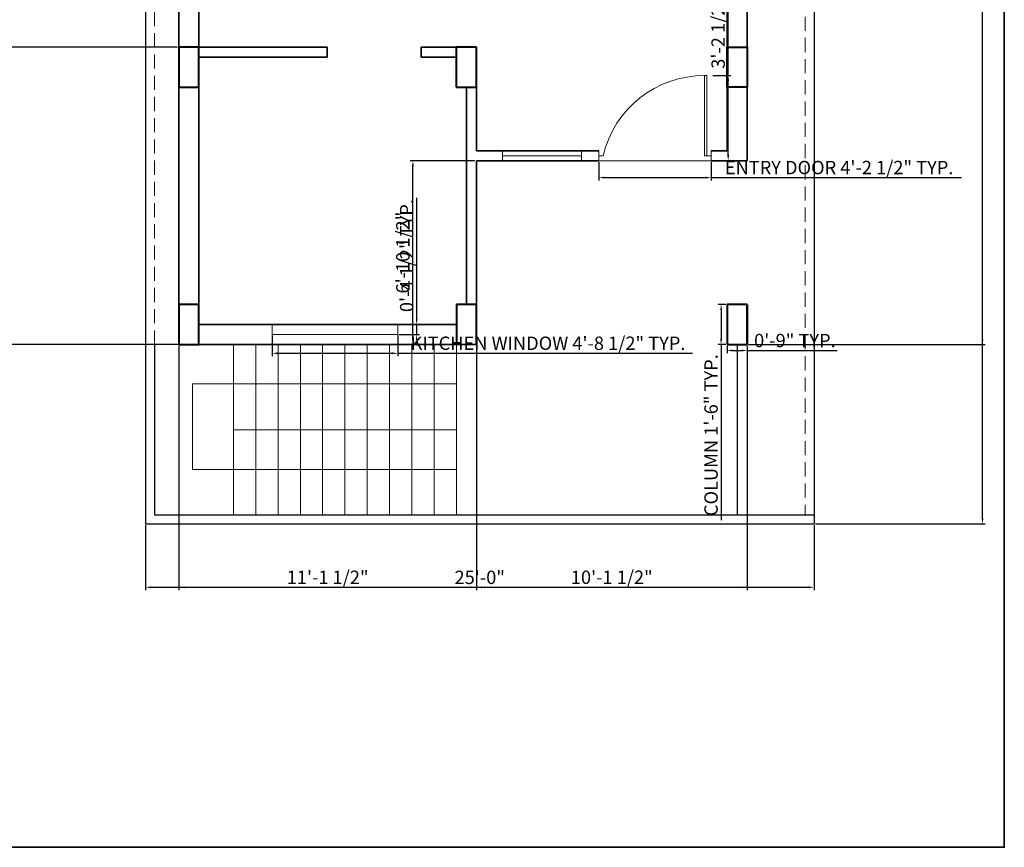
# Model space of a CAD drawing. Units: inches. Extents: x 2656 to 9931, y 1941 to 3068.
# Tile 26 of 46: x 3074 to 3515, y 1941 to 2312. Entities that reach past the tile are written whole.
import ezdxf

# ---------------------------------------------------------------- set-up
doc = ezdxf.new("R2010")
doc.units = ezdxf.units.IN
doc.linetypes.add('DASHED2', pattern=[9.525, 6.35, -3.175])
for name, color, linetype, lineweight in [('A-ANNO-DIMS', 2, 'Continuous', 18), ('A-ANNO-TTLB', 7, 'Continuous', 35), ('A-COLS', 7, 'Continuous', 40), ('A-DOOR', 3, 'Continuous', 18), ('A-FLOR-OVHD', 252, 'DASHED2', 13), ('A-FLOR-STRS', 7, 'Continuous', 18), ('A-GLAZ', 4, 'Continuous', 18), ('A-WALL', 7, 'Continuous', 35), ('C-PROP', 7, 'Continuous', 25)]:
    doc.layers.add(name, color=color, linetype=linetype, lineweight=lineweight)
doc.styles.get("Standard").update_dxf_attribs({"font": 'arial.ttf'})
doc.dimstyles.new('ISO-25', dxfattribs={"dimtxt": 6, "dimasz": 2.5, "dimexe": 1.25, "dimexo": 0.625, "dimtad": 1, "dimdec": 0, "dimlunit": 3, "dimtxsty": 'Standard', "dimcen": 2.5, "dimadec": 0, "dimazin": 0, "dimtfac": 1, "dimtdec": 0, "dimtmove": 0, "dimatfit": 3, "dimfxl": 1, "dimarcsym": 0})

# ---------------------------------------------------------------- blocks, each defined once
blk = doc.blocks.new('DOOR-ENTRY')
for p, q in [((48.56, 38.25), (47.56, 38.25)), ((47.56, 38.25), (47.56, 2.25)), ((48.56, 2.25), (48.56, 38.25)), ((0.04, 2.25), (2.04, 2.25)), ((0.04, 0), (50.56, 0)), ((47.56, 2.25), (48.56, 2.25)), ((50.56, 2.25), (48.56, 2.25))]:
    blk.add_line(p, q)
blk.add_arc((47.56, -8.52), 46.77, 90, 166.6828)
blk = doc.blocks.new('WIN-ENTRY')
for p, q in [((35.5, -0.05), (35.5, 2.2)), ((0.02, -0.05), (35.5, -0.05))]:
    blk.add_line(p, q)
blk = doc.blocks.new('WIN-KITCHEN')
for p, q in [((56.32, 0), (56.32, 4.5)), ((-0.04, 0), (56.32, 0))]:
    blk.add_line(p, q)
blk = doc.blocks.new('STAIR-FRONT')
for p, q in [((28.36, 76.5), (18.36, 76.5)), ((18.36, 76.5), (18.36, 0)), ((28.36, 76.5), (28.36, 0)), ((38.36, 76.5), (38.36, 0)), ((48.36, 76.5), (48.36, 0)), ((58.36, 76.5), (58.36, 0)), ((68.36, 76.5), (68.36, 0)), ((78.36, 76.5), (78.36, 0)), ((88.36, 76.5), (88.36, 0)), ((98.36, 76.5), (98.36, 0)), ((108.36, 76.5), (108.36, 0)), ((118.36, 76.5), (118.36, 0)), ((118.36, 58.83), (-0.04, 58.83)), ((-0.04, 58.83), (-0.04, 20.36)), ((18.36, 0), (18.36, 38.25)), ((18.36, 38.25), (28.36, 38.25)), ((118.36, 38.25), (28.36, 38.25)), ((118.36, 0), (118.36, 38.25)), ((-0.04, 20.36), (118.36, 20.36))]:
    blk.add_line(p, q)
blk = doc.blocks.new('COL-9X18')
for p, q in [((18.05, 9), (0.05, 9)), ((0.05, 9), (0.05, 0)), ((18.05, 0), (18.05, 9)), ((0.05, 0), (18.05, 0))]:
    blk.add_line(p, q)
blk = doc.blocks.new('*D25')
at = {"layer": 'A-ANNO-DIMS', "color": 0, "lineweight": -2, "transparency": 16777216}
for p, q in [((3390.42, 2184.6), (3387.1, 2184.6)), ((3388.35, 2182.1), (3388.35, 2169.1)), ((3390.42, 2166.6), (3387.1, 2166.6)), ((3388.35, 2166.6), (3388.35, 2087.69))]:
    blk.add_line(p, q, dxfattribs=at)
at = {"layer": 'A-ANNO-DIMS', "color": 0, "transparency": 16777216}
for points in [[(3387.93, 2182.1), (3388.76, 2182.1), (3388.35, 2184.6)], [(3387.93, 2169.1), (3388.76, 2169.1), (3388.35, 2166.6)]]:
    blk.add_solid(points, dxfattribs=at)
at = {"layer": 'Defpoints', "color": 0, "transparency": 16777216}
for p in [(3391.05, 2184.6), (3388.35, 2166.6), (3391.05, 2166.6)]:
    blk.add_point(p, dxfattribs=at)
at = {"layer": 'A-ANNO-DIMS', "color": 0, "transparency": 16777216, "insert": (3384.62, 2125.9), "char_height": 6, "attachment_point": 5, "rotation": 90}
blk.add_mtext('COLUMN 1\'-6" TYP.', dxfattribs=at)
blk = doc.blocks.new('*D26')
at = {"layer": 'A-ANNO-DIMS', "color": 0, "lineweight": -2, "transparency": 16777216}
for p, q in [((3391.05, 2165.98), (3391.05, 2162.65)), ((3400.05, 2165.98), (3400.05, 2162.65)), ((3393.55, 2163.9), (3397.55, 2163.9)), ((3400.05, 2163.9), (3440.37, 2163.9))]:
    blk.add_line(p, q, dxfattribs=at)
at = {"layer": 'A-ANNO-DIMS', "color": 0, "transparency": 16777216}
for points in [[(3393.55, 2164.32), (3393.55, 2163.48), (3391.05, 2163.9)], [(3397.55, 2164.32), (3397.55, 2163.48), (3400.05, 2163.9)]]:
    blk.add_solid(points, dxfattribs=at)
at = {"layer": 'Defpoints', "color": 0, "transparency": 16777216}
for p in [(3391.05, 2166.6), (3400.05, 2166.6), (3400.05, 2163.9)]:
    blk.add_point(p, dxfattribs=at)
at = {"layer": 'A-ANNO-DIMS', "color": 0, "transparency": 16777216, "insert": (3421.46, 2167.59), "char_height": 6, "attachment_point": 5}
blk.add_mtext('0\'-9" TYP.', dxfattribs=at)
blk = doc.blocks.new('*D41')
at = {"layer": 'A-ANNO-DIMS', "color": 0, "lineweight": -2, "transparency": 16777216}
for p, q in [((3333.43, 2248.48), (3333.43, 2240.27)), ((3383.95, 2248.48), (3383.95, 2240.27)), ((3335.93, 2241.52), (3381.45, 2241.52)), ((3383.95, 2241.52), (3496.15, 2241.52))]:
    blk.add_line(p, q, dxfattribs=at)
at = {"layer": 'A-ANNO-DIMS', "color": 0, "transparency": 16777216}
for points in [[(3335.93, 2241.94), (3335.93, 2241.11), (3333.43, 2241.52)], [(3381.45, 2241.94), (3381.45, 2241.11), (3383.95, 2241.52)]]:
    blk.add_solid(points, dxfattribs=at)
at = {"layer": 'Defpoints', "color": 0, "transparency": 16777216}
for p in [(3333.43, 2249.1), (3383.95, 2249.1), (3383.95, 2241.52)]:
    blk.add_point(p, dxfattribs=at)
at = {"layer": 'A-ANNO-DIMS', "color": 0, "transparency": 16777216, "insert": (3441.3, 2245.25), "char_height": 6, "attachment_point": 5}
blk.add_mtext('ENTRY DOOR 4\'-2 1/2" TYP.', dxfattribs=at)
blk = doc.blocks.new('*D42')
at = {"layer": 'A-ANNO-DIMS', "color": 0, "lineweight": -2, "transparency": 16777216}
for p, q in [((3391.52, 2287.35), (3391.52, 2341.65)), ((3384.57, 2287.35), (3392.77, 2287.35)), ((3391.52, 2251.6), (3391.52, 2284.85)), ((3384.57, 2249.1), (3392.77, 2249.1))]:
    blk.add_line(p, q, dxfattribs=at)
at = {"layer": 'A-ANNO-DIMS', "color": 0, "transparency": 16777216}
for points in [[(3391.11, 2284.85), (3391.94, 2284.85), (3391.52, 2287.35)], [(3391.11, 2251.6), (3391.94, 2251.6), (3391.52, 2249.1)]]:
    blk.add_solid(points, dxfattribs=at)
at = {"layer": 'Defpoints', "color": 0, "transparency": 16777216}
for p in [(3383.95, 2287.35), (3391.52, 2287.35), (3383.95, 2249.1)]:
    blk.add_point(p, dxfattribs=at)
at = {"layer": 'A-ANNO-DIMS', "color": 0, "transparency": 16777216, "insert": (3387.79, 2315.75), "char_height": 6, "attachment_point": 5, "rotation": 90}
blk.add_mtext('3\'-2 1/2" TYP.', dxfattribs=at)
blk = doc.blocks.new('*D51')
at = {"layer": 'A-ANNO-DIMS', "color": 0, "lineweight": -2, "transparency": 16777216}
for p, q in [((3186.95, 2170.48), (3186.95, 2161.4)), ((3243.31, 2170.48), (3243.31, 2161.4)), ((3189.45, 2162.65), (3240.81, 2162.65)), ((3243.31, 2162.65), (3375.57, 2162.65))]:
    blk.add_line(p, q, dxfattribs=at)
at = {"layer": 'A-ANNO-DIMS', "color": 0, "transparency": 16777216}
for points in [[(3189.45, 2163.06), (3189.45, 2162.23), (3186.95, 2162.65)], [(3240.81, 2163.06), (3240.81, 2162.23), (3243.31, 2162.65)]]:
    blk.add_solid(points, dxfattribs=at)
at = {"layer": 'Defpoints', "color": 0, "transparency": 16777216}
for p in [(3186.95, 2171.1), (3243.31, 2171.1), (3243.31, 2162.65)]:
    blk.add_point(p, dxfattribs=at)
at = {"layer": 'A-ANNO-DIMS', "color": 0, "transparency": 16777216, "insert": (3310.69, 2166.38), "char_height": 6, "attachment_point": 5}
blk.add_mtext('KITCHEN WINDOW 4\'-8 1/2" TYP.', dxfattribs=at)
blk = doc.blocks.new('*D52')
at = {"layer": 'A-ANNO-DIMS', "color": 0, "lineweight": -2, "transparency": 16777216}
for p, q in [((3251.76, 2178.1), (3251.76, 2232.4)), ((3243.93, 2175.6), (3253.01, 2175.6)), ((3251.76, 2171.1), (3251.76, 2175.6)), ((3243.93, 2171.1), (3253.01, 2171.1)), ((3251.76, 2168.6), (3251.76, 2166.1))]:
    blk.add_line(p, q, dxfattribs=at)
at = {"layer": 'A-ANNO-DIMS', "color": 0, "transparency": 16777216}
for points in [[(3251.34, 2178.1), (3252.18, 2178.1), (3251.76, 2175.6)], [(3251.34, 2168.6), (3252.18, 2168.6), (3251.76, 2171.1)]]:
    blk.add_solid(points, dxfattribs=at)
at = {"layer": 'Defpoints', "color": 0, "transparency": 16777216}
for p in [(3243.31, 2175.6), (3251.76, 2175.6), (3243.31, 2171.1)]:
    blk.add_point(p, dxfattribs=at)
at = {"layer": 'A-ANNO-DIMS', "color": 0, "transparency": 16777216, "insert": (3248.03, 2206.5), "char_height": 6, "attachment_point": 5, "rotation": 90}
blk.add_mtext('0\'-4 1/2" TYP.', dxfattribs=at)
blk = doc.blocks.new('*D66')
at = {"layer": 'A-ANNO-DIMS', "color": 0, "lineweight": -2, "transparency": 16777216}
for p, q in [((3400.67, 2623.6), (3506.9, 2623.6)), ((3505.65, 2169.1), (3505.65, 2621.1)), ((3400.67, 2166.6), (3506.9, 2166.6))]:
    blk.add_line(p, q, dxfattribs=at)
at = {"layer": 'A-ANNO-DIMS', "color": 0, "transparency": 16777216}
for points in [[(3505.23, 2621.1), (3506.07, 2621.1), (3505.65, 2623.6)], [(3505.23, 2169.1), (3506.07, 2169.1), (3505.65, 2166.6)]]:
    blk.add_solid(points, dxfattribs=at)
at = {"layer": 'Defpoints', "color": 0, "transparency": 16777216}
for p in [(3400.05, 2623.6), (3505.65, 2623.6), (3400.05, 2166.6)]:
    blk.add_point(p, dxfattribs=at)
at = {"layer": 'A-ANNO-DIMS', "color": 0, "transparency": 16777216, "insert": (3501.96, 2395.1), "char_height": 6, "attachment_point": 5, "rotation": 90}
blk.add_mtext('38\'-1"', dxfattribs=at)
blk = doc.blocks.new('*D67')
at = {"layer": 'A-ANNO-DIMS', "color": 0, "lineweight": -2, "transparency": 16777216}
for p, q in [((3145.05, 2165.98), (3145.05, 2056.35)), ((3278.55, 2165.98), (3278.55, 2056.35)), ((3147.55, 2057.6), (3276.05, 2057.6))]:
    blk.add_line(p, q, dxfattribs=at)
at = {"layer": 'A-ANNO-DIMS', "color": 0, "transparency": 16777216}
for points in [[(3147.55, 2058.02), (3147.55, 2057.18), (3145.05, 2057.6)], [(3276.05, 2058.02), (3276.05, 2057.18), (3278.55, 2057.6)]]:
    blk.add_solid(points, dxfattribs=at)
at = {"layer": 'Defpoints', "color": 0, "transparency": 16777216}
for p in [(3145.05, 2166.6), (3278.55, 2166.6), (3278.55, 2057.6)]:
    blk.add_point(p, dxfattribs=at)
at = {"layer": 'A-ANNO-DIMS', "color": 0, "transparency": 16777216, "insert": (3211.8, 2061.33), "char_height": 6, "attachment_point": 5}
blk.add_mtext('11\'-1 1/2"', dxfattribs=at)
blk = doc.blocks.new('*D68')
at = {"layer": 'A-ANNO-DIMS', "color": 0, "lineweight": -2, "transparency": 16777216}
for p, q in [((3278.55, 2165.98), (3278.55, 2056.35)), ((3400.05, 2165.98), (3400.05, 2056.35)), ((3281.05, 2057.6), (3397.55, 2057.6))]:
    blk.add_line(p, q, dxfattribs=at)
at = {"layer": 'A-ANNO-DIMS', "color": 0, "transparency": 16777216}
for points in [[(3281.05, 2058.02), (3281.05, 2057.18), (3278.55, 2057.6)], [(3397.55, 2058.02), (3397.55, 2057.18), (3400.05, 2057.6)]]:
    blk.add_solid(points, dxfattribs=at)
at = {"layer": 'Defpoints', "color": 0, "transparency": 16777216}
for p in [(3278.55, 2166.6), (3400.05, 2166.6), (3400.05, 2057.6)]:
    blk.add_point(p, dxfattribs=at)
at = {"layer": 'A-ANNO-DIMS', "color": 0, "transparency": 16777216, "insert": (3339.3, 2061.33), "char_height": 6, "attachment_point": 5}
blk.add_mtext('10\'-1 1/2"', dxfattribs=at)
blk = doc.blocks.new('*D69')
at = {"layer": 'A-ANNO-DIMS', "color": 0, "lineweight": -2, "transparency": 16777216}
for p, q in [((3144.42, 2300.1), (3052.46, 2300.1)), ((3053.71, 2169.1), (3053.71, 2297.6)), ((3144.42, 2166.6), (3052.46, 2166.6))]:
    blk.add_line(p, q, dxfattribs=at)
at = {"layer": 'A-ANNO-DIMS', "color": 0, "transparency": 16777216}
for points in [[(3053.3, 2297.6), (3054.13, 2297.6), (3053.71, 2300.1)], [(3053.3, 2169.1), (3054.13, 2169.1), (3053.71, 2166.6)]]:
    blk.add_solid(points, dxfattribs=at)
at = {"layer": 'Defpoints', "color": 0, "transparency": 16777216}
for p in [(3053.71, 2300.1), (3145.05, 2300.1), (3145.05, 2166.6)]:
    blk.add_point(p, dxfattribs=at)
at = {"layer": 'A-ANNO-DIMS', "color": 0, "transparency": 16777216, "insert": (3049.99, 2233.35), "char_height": 6, "attachment_point": 5, "rotation": 90}
blk.add_mtext('11\'-1 1/2"', dxfattribs=at)
blk = doc.blocks.new('*D70')
at = {"layer": 'A-ANNO-DIMS', "color": 0, "lineweight": -2, "transparency": 16777216}
for p, q in [((3088.25, 2342.93), (3052.46, 2342.93)), ((3053.71, 2302.6), (3053.71, 2340.43)), ((3144.42, 2300.1), (3052.46, 2300.1))]:
    blk.add_line(p, q, dxfattribs=at)
at = {"layer": 'A-ANNO-DIMS', "color": 0, "transparency": 16777216}
for points in [[(3053.3, 2340.43), (3054.13, 2340.43), (3053.71, 2342.93)], [(3053.3, 2302.6), (3054.13, 2302.6), (3053.71, 2300.1)]]:
    blk.add_solid(points, dxfattribs=at)
at = {"layer": 'Defpoints', "color": 0, "transparency": 16777216}
for p in [(3053.71, 2342.93), (3088.87, 2342.93), (3145.05, 2300.1)]:
    blk.add_point(p, dxfattribs=at)
at = {"layer": 'A-ANNO-DIMS', "color": 0, "transparency": 16777216, "insert": (3050.02, 2321.51), "char_height": 6, "attachment_point": 5, "rotation": 90}
blk.add_mtext('3\'-7"', dxfattribs=at)
blk = doc.blocks.new('*D172')
at = {"layer": 'A-ANNO-DIMS', "color": 0, "lineweight": -2, "transparency": 16777216}
for p, q in [((3130.05, 2085.48), (3130.05, 2056.35)), ((3430.05, 2085.48), (3430.05, 2056.35)), ((3132.55, 2057.6), (3427.55, 2057.6))]:
    blk.add_line(p, q, dxfattribs=at)
at = {"layer": 'A-ANNO-DIMS', "color": 0, "transparency": 16777216}
for points in [[(3132.55, 2058.02), (3132.55, 2057.18), (3130.05, 2057.6)], [(3427.55, 2058.02), (3427.55, 2057.18), (3430.05, 2057.6)]]:
    blk.add_solid(points, dxfattribs=at)
at = {"layer": 'Defpoints', "color": 0, "transparency": 16777216}
for p in [(3130.05, 2086.1), (3430.05, 2086.1), (3430.05, 2057.6)]:
    blk.add_point(p, dxfattribs=at)
at = {"layer": 'A-ANNO-DIMS', "color": 0, "transparency": 16777216, "insert": (3280.05, 2061.29), "char_height": 6, "attachment_point": 5}
blk.add_mtext('25\'-0"', dxfattribs=at)
blk = doc.blocks.new('*D173')
at = {"layer": 'A-ANNO-DIMS', "color": 0, "lineweight": -2, "transparency": 16777216}
for p, q in [((3430.67, 2641.6), (3506.9, 2641.6)), ((3505.65, 2088.6), (3505.65, 2639.1)), ((3430.67, 2086.1), (3506.9, 2086.1))]:
    blk.add_line(p, q, dxfattribs=at)
at = {"layer": 'A-ANNO-DIMS', "color": 0, "transparency": 16777216}
for points in [[(3505.23, 2639.1), (3506.07, 2639.1), (3505.65, 2641.6)], [(3505.23, 2088.6), (3506.07, 2088.6), (3505.65, 2086.1)]]:
    blk.add_solid(points, dxfattribs=at)
at = {"layer": 'Defpoints', "color": 0, "transparency": 16777216}
for p in [(3430.05, 2641.6), (3505.65, 2641.6), (3430.05, 2086.1)]:
    blk.add_point(p, dxfattribs=at)
at = {"layer": 'A-ANNO-DIMS', "color": 0, "transparency": 16777216, "insert": (3501.92, 2363.85), "char_height": 6, "attachment_point": 5, "rotation": 90}
blk.add_mtext('46\'-3 1/2"', dxfattribs=at)
blk = doc.blocks.new('*D178')
at = {"layer": 'A-ANNO-DIMS', "color": 0, "lineweight": -2, "transparency": 16777216}
for p, q in [((3277.92, 2249.1), (3248.8, 2249.1)), ((3250.05, 2169.1), (3250.05, 2246.6)), ((3277.92, 2166.6), (3248.8, 2166.6))]:
    blk.add_line(p, q, dxfattribs=at)
at = {"layer": 'A-ANNO-DIMS', "color": 0, "transparency": 16777216}
for points in [[(3249.63, 2246.6), (3250.46, 2246.6), (3250.05, 2249.1)], [(3249.63, 2169.1), (3250.46, 2169.1), (3250.05, 2166.6)]]:
    blk.add_solid(points, dxfattribs=at)
at = {"layer": 'Defpoints', "color": 0, "transparency": 16777216}
for p in [(3250.05, 2249.1), (3278.55, 2249.1), (3278.55, 2166.6)]:
    blk.add_point(p, dxfattribs=at)
at = {"layer": 'A-ANNO-DIMS', "color": 0, "transparency": 16777216, "insert": (3246.32, 2207.85), "char_height": 6, "attachment_point": 5, "rotation": 90}
blk.add_mtext('6\'-10 1/2"', dxfattribs=at)

msp = doc.modelspace()

# ---------------------------------------------------------------- linework, layer by layer
at = {"layer": 'A-ANNO-TTLB'}
msp.add_lwpolyline([(2655.77, 3067.84), (3515.43, 3067.84), (3515.43, 1940.89), (2655.77, 1940.89)], close=True, dxfattribs=at)
at = {"layer": 'A-COLS'}
for p, q in [((3391.05, 2300.1), (3400.05, 2300.1)), ((3391.05, 2282.1), (3391.05, 2300.1)), ((3400.05, 2300.1), (3400.05, 2282.1)), ((3400.05, 2282.1), (3391.05, 2282.1)), ((3391.05, 2282.1), (3391.05, 2282.1)), ((3278.55, 2184.6), (3269.55, 2184.6)), ((3269.55, 2184.6), (3269.55, 2166.6)), ((3278.55, 2166.6), (3278.55, 2184.6)), ((3391.05, 2184.6), (3391.05, 2166.6)), ((3400.05, 2184.6), (3400.05, 2166.6)), ((3391.05, 2166.6), (3400.05, 2166.6))]:
    msp.add_line(p, q, dxfattribs=at)
at = {"layer": 'A-DOOR'}
for p, q in [((3333.43, 2253.6), (3333.43, 2249.1)), ((3383.95, 2253.6), (3383.95, 2249.1))]:
    msp.add_line(p, q, dxfattribs=at)
at = {"layer": 'A-FLOR-OVHD'}
for p, q in [((3134.05, 2166.6), (3134.05, 2637.6)), ((3426.05, 2637.6), (3426.05, 2090.1)), ((3134.05, 2166.6), (3134.05, 2173.4)), ((3145.05, 2166.6), (3134.05, 2166.6))]:
    msp.add_line(p, q, dxfattribs=at)
at = {"layer": 'A-GLAZ'}
for p, q in [((3290.21, 2253.6), (3290.21, 2249.1)), ((3325.68, 2253.6), (3325.68, 2249.1)), ((3290.21, 2249.1), (3290.21, 2251.35)), ((3186.95, 2175.6), (3186.95, 2166.6)), ((3243.31, 2175.6), (3243.31, 2166.6)), ((3186.95, 2166.6), (3186.95, 2171.1))]:
    msp.add_line(p, q, dxfattribs=at)
at = {"layer": 'A-WALL'}
for p, q in [((3145.05, 2623.6), (3145.05, 2166.6)), ((3400.05, 2623.6), (3400.05, 2249.1)), ((3154.05, 2614.6), (3154.05, 2166.6)), ((3391.05, 2385.6), (3391.05, 2253.6)), ((3154.05, 2300.1), (3211.66, 2300.1)), ((3211.66, 2300.1), (3211.66, 2295.6)), ((3253.76, 2300.1), (3278.55, 2300.1)), ((3253.76, 2300.1), (3253.76, 2295.6)), ((3278.55, 2300.1), (3278.55, 2253.6)), ((3154.05, 2295.6), (3211.66, 2295.6)), ((3253.76, 2295.6), (3269.55, 2295.6)), ((3274.05, 2282.1), (3274.05, 2184.6)), ((3278.55, 2253.6), (3333.43, 2253.6)), ((3383.95, 2253.6), (3391.05, 2253.6)), ((3278.55, 2249.1), (3278.55, 2166.6)), ((3278.55, 2249.1), (3333.43, 2249.1)), ((3383.95, 2249.1), (3391.05, 2249.1)), ((3391.05, 2249.1), (3400.05, 2249.1)), ((3154.05, 2175.6), (3269.55, 2175.6)), ((3145.05, 2166.6), (3278.55, 2166.6))]:
    msp.add_line(p, q, dxfattribs=at)
at = {"layer": 'C-PROP'}
for p, q in [((3130.05, 2641.6), (3130.05, 2086.1)), ((3430.05, 2641.6), (3430.05, 2086.1)), ((3134.05, 2166.6), (3134.05, 2090.1)), ((3395.55, 2166.6), (3395.55, 2090.1)), ((3134.05, 2090.1), (3430.05, 2090.1)), ((3130.05, 2086.1), (3430.05, 2086.1))]:
    msp.add_line(p, q, dxfattribs=at)

# ---------------------------------------------------------------- block references
at = {"layer": 'A-COLS'}
for p, rotation in [((3145.04, 2300.15), 269.9999999999988), ((3269.54, 2300.15), 269.9999999999965), ((3154.05, 2166.56), 89.99999999999422), ((3391.04, 2184.65), 269.9999999999988)]:
    msp.add_blockref('COL-9X18', p, dxfattribs=dict(at, rotation=rotation))
at = {"layer": 'A-DOOR'}
msp.add_blockref('DOOR-ENTRY', (3333.39, 2249.1), dxfattribs=at)
at = {"layer": 'A-FLOR-STRS'}
msp.add_blockref('STAIR-FRONT', (3151.19, 2090.1), dxfattribs=at)
at = {"layer": 'A-GLAZ'}
for name, p in [('WIN-ENTRY', (3290.19, 2251.4)), ('WIN-KITCHEN', (3186.99, 2171.1))]:
    msp.add_blockref(name, p, dxfattribs=at)

# ---------------------------------------------------------------- dimensions: what is measured, and where the dimension line sits
at = {"layer": 'A-ANNO-DIMS'}
for base, p1, p2, picture, middle in [((3505.65, 2641.6), (3430.05, 2086.1), (3430.05, 2641.6), '*D173', (3501.92, 2363.85)), ((3505.65, 2623.6), (3400.05, 2166.6), (3400.05, 2623.6), '*D66', (3501.96, 2395.1)), ((3053.71, 2342.93), (3145.05, 2300.1), (3088.87, 2342.93), '*D70', (3050.02, 2321.51)), ((3053.71, 2300.1), (3145.05, 2166.6), (3145.05, 2300.1), '*D69', (3049.99, 2233.35)), ((3250.05, 2249.1), (3278.55, 2166.6), (3278.55, 2249.1), '*D178', (3246.32, 2207.85))]:
    dim = msp.add_linear_dim(base=base, p1=p1, p2=p2, angle=90, dimstyle='ISO-25', override={"dimdec": 1, "dimlfac": 1, "dimrnd": 0, "dimzin": 1, "dimdsep": 46, "dimlunit": 4, "dimfrac": 2}, dxfattribs=at)
    dim.commit()
    dim.dimension.update_dxf_attribs({"geometry": picture, "text_midpoint": middle})
for base, p1, p2, angle, text, picture, middle in [((3391.52361648, 2287.35027301), (3383.94617811, 2249.10027301), (3383.94617811, 2287.35027301), 90, '<> TYP.', '*D42', (3387.79425086, 2315.75017069)), ((3251.76, 2175.6), (3243.31, 2171.1), (3243.31, 2175.6), 90, '<> TYP.', '*D52', (3248.03, 2206.5)), ((3388.35, 2166.6), (3391.05, 2184.6), (3391.05, 2166.6), 270, 'COLUMN <> TYP.', '*D25', (3384.62, 2125.9))]:
    dim = msp.add_linear_dim(base=base, p1=p1, p2=p2, angle=angle, text=text, dimstyle='ISO-25', override={"dimdec": 1, "dimlfac": 1, "dimrnd": 0, "dimzin": 1, "dimdsep": 46, "dimlunit": 4, "dimfrac": 2}, dxfattribs=at)
    dim.commit()
    dim.dimension.update_dxf_attribs({"geometry": picture, "text_midpoint": middle})
for base, p1, p2, text, picture, middle in [((3383.95, 2241.52), (3333.43, 2249.1), (3383.95, 2249.1), 'ENTRY DOOR <> TYP.', '*D41', (3441.3, 2245.25)), ((3243.31, 2162.65), (3186.95, 2171.1), (3243.31, 2171.1), 'KITCHEN WINDOW <> TYP.', '*D51', (3310.69, 2166.38)), ((3400.05, 2163.9), (3391.05, 2166.6), (3400.05, 2166.6), '<> TYP.', '*D26', (3421.46, 2167.59))]:
    dim = msp.add_linear_dim(base=base, p1=p1, p2=p2, text=text, dimstyle='ISO-25', override={"dimdec": 1, "dimlfac": 1, "dimrnd": 0, "dimzin": 1, "dimdsep": 46, "dimlunit": 4, "dimfrac": 2}, dxfattribs=at)
    dim.commit()
    dim.dimension.update_dxf_attribs({"geometry": picture, "text_midpoint": middle})
for base, p1, p2, picture, middle in [((3278.55, 2057.6), (3145.05, 2166.6), (3278.55, 2166.6), '*D67', (3211.8, 2061.33)), ((3400.05, 2057.6), (3278.55, 2166.6), (3400.05, 2166.6), '*D68', (3339.3, 2061.33)), ((3430.05, 2057.6), (3130.05, 2086.1), (3430.05, 2086.1), '*D172', (3280.05, 2061.29))]:
    dim = msp.add_linear_dim(base=base, p1=p1, p2=p2, dimstyle='ISO-25', override={"dimdec": 1, "dimlfac": 1, "dimrnd": 0, "dimzin": 1, "dimdsep": 46, "dimlunit": 4, "dimfrac": 2}, dxfattribs=at)
    dim.commit()
    dim.dimension.update_dxf_attribs({"geometry": picture, "text_midpoint": middle})

doc.saveas('drawing.dxf')
